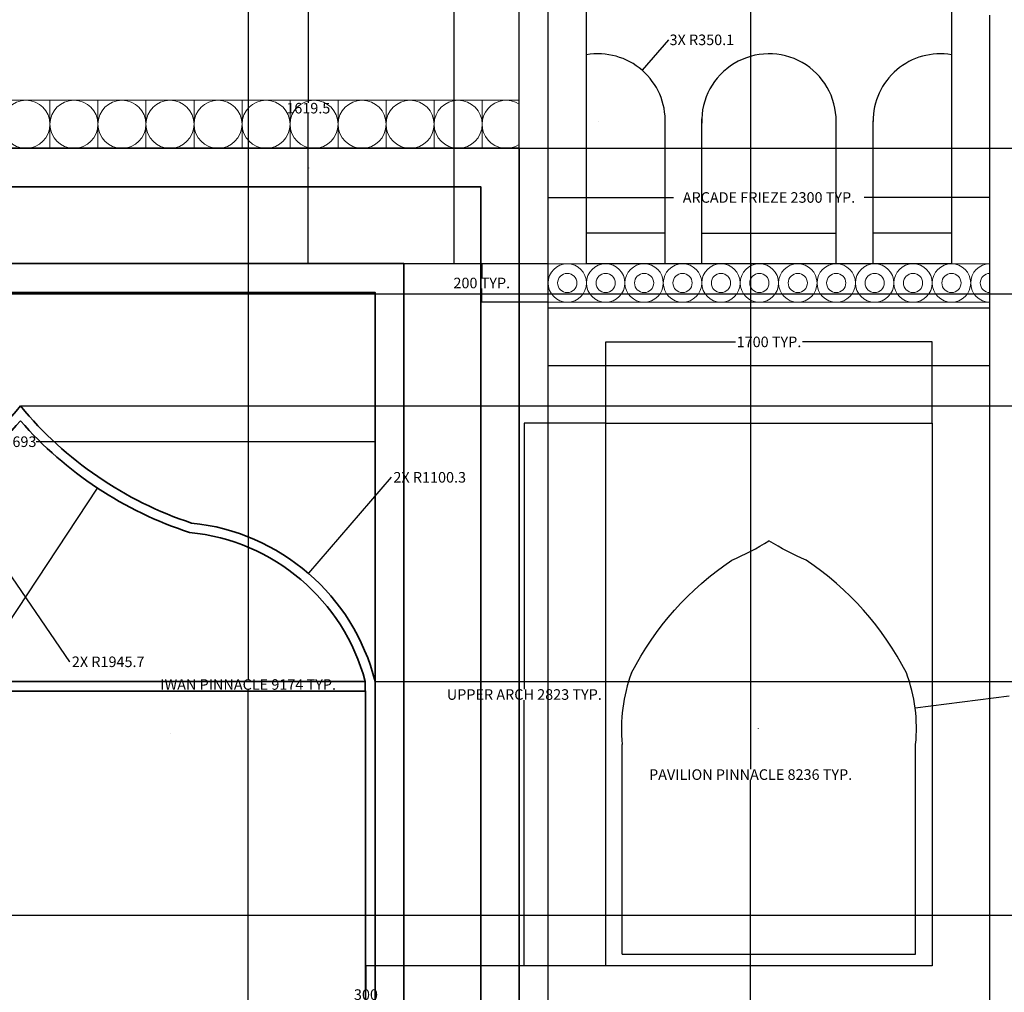
# Model space of a CAD drawing. Units: millimetres. Extents: x 8570 to 49085, y 3782 to 24863.
# Tile 6 of 15: x 22404 to 27529, y 10208 to 15269. Entities that reach past the tile are written whole.
import ezdxf

# ---------------------------------------------------------------- set-up
doc = ezdxf.new("R2010")
doc.units = ezdxf.units.MM
doc.header["$MEASUREMENT"] = 0
doc.header["$PDMODE"] = 3
for name, color, linetype, lineweight in [('A-ANNO-DIMS', 2, 'Continuous', 18), ('A-ELEV', 7, 'Continuous', 25), ('A-ELEV-ARCH', 7, 'Continuous', 25), ('A-ELEV-IWAN', 7, 'Continuous', 35), ('A-ELEV-ORNM', 7, 'Continuous', 13), ('A-ELEV-PIER', 7, 'Continuous', 25), ('A-ROOF-CHAT', 7, 'Continuous', 25)]:
    doc.layers.add(name, color=color, linetype=linetype, lineweight=lineweight)
doc.styles.get("Standard").update_dxf_attribs({"font": 'arial.ttf'})
doc.dimstyles.get("Standard").update_dxf_attribs({"dimtxt": 55, "dimasz": 0.18, "dimexe": 0.18, "dimexo": 0.0625, "dimgap": 0.09, "dimtad": 0, "dimtih": 1, "dimtoh": 1, "dimdec": 0, "dimzin": 0, "dimdsep": 46, "dimtxsty": 'Standard', "dimcen": 0.09, "dimadec": 0, "dimazin": 0, "dimtfac": 1, "dimtdec": 0, "dimtofl": 0, "dimtmove": 0, "dimatfit": 3, "dimfxl": 1, "dimtolj": 1, "dimtzin": 0, "dimarcsym": 0})

# ---------------------------------------------------------------- blocks, each defined once
blk = doc.blocks.new('IWAN-EDGE-PINNACLE')
for p, q in [((35, 0), (35, 9004.5)), ((185, 0), (185, 9004.5))]:
    blk.add_line(p, q)
blk = doc.blocks.new('PAVILION-EDGE-PINNACLE')
for q in [(10, 8069.5), (10, 6246.5)]:
    blk.add_line((10, 0), q)
blk = doc.blocks.new('ARCADE-RING-FRIEZE')
for p, q in [((0, 200), (2300, 200)), ((2300, 200), (2100, 200)), ((0, 0), (2300, 0))]:
    blk.add_line(p, q)
for centre, radius in [((100, 100), 100), ((300, 100), 100), ((500, 100), 100), ((700, 100), 100), ((900, 100), 100), ((1100, 100), 100), ((1300, 100), 100), ((1500, 100), 100), ((1700, 100), 100), ((1900, 100), 100), ((2100, 100), 100), ((100, 100), 50), ((300, 100), 50), ((500, 100), 50), ((700, 100), 50), ((900, 100), 50), ((1100, 100), 50), ((1300, 100), 50), ((1500, 100), 50), ((1700, 100), 50), ((1900, 100), 50), ((2100, 100), 50)]:
    blk.add_circle(centre, radius)
for radius in [100, 50]:
    blk.add_arc((2300, 100), radius, 90, 270)
blk = doc.blocks.new('CHHATRI-ELEV')
for p, q in [((1107.1, 3111.9), (1194.6, 3111.9)), ((819.3, 2507.3), (1150, 2958.1)), ((967.4, 2449.5), (1150, 2958.1)), ((1480.7, 2507.3), (1150, 2958.1)), ((1339.8, 2454.2), (1150, 2958.1)), ((200, 1639.5), (2100, 1639.5)), ((2300, 1569.5), (2300, 1619.5)), ((200, 1549.5), (2100, 1549.5)), ((610, 0), (610, 754)), ((800, 0), (800, 754)), ((1500, 0), (1500, 744.5)), ((1692, 0), (1692, 744.5)), ((610, 158.5), (200, 158.5)), ((800, 158.5), (1500, 158.5)), ((2100, 158.5), (1692, 158.5))]:
    blk.add_line(p, q)
for points in [[(1199.3, 3183.7, 0.216309), (1151.6, 3264, 0.244698), (1103.6, 3171.4, 0.244698)], [(1198.5, 3007.8, 0.216309), (1150.8, 3088.1, 0.244698), (1102.8, 2995.4, 0.244698)], [(259.6, 2102.5, -0.128405), (908.9, 2832.4, 0.03556), (1150, 2958.1)], [(2040.4, 2102.5, 0.128405), (1391.1, 2832.4, -0.03556), (1150, 2958.1)]]:
    blk.add_lwpolyline(points, format="xyb")
for points in [[(225.8, 1639.5, 0.520567), (200.9, 1667.5, 0.520567)], [(273.9, 1639.5, 0.520567), (249, 1667.5, 0.520567)], [(321.9, 1639.5, 0.520567), (297.1, 1667.5, 0.520567)], [(370, 1639.5, 0.520567), (345.1, 1667.5, 0.520567)], [(418, 1639.5, 0.520567), (393.2, 1667.5, 0.520567)], [(466.1, 1639.5, 0.520567), (441.2, 1667.5, 0.520567)], [(514.2, 1639.5, 0.520567), (489.3, 1667.5, 0.520567)], [(562.2, 1639.5, 0.520567), (537.3, 1667.5, 0.520567)], [(610.3, 1639.5, 0.520567), (585.4, 1667.5, 0.520567)], [(658.3, 1639.5, 0.520567), (633.4, 1667.5, 0.520567)], [(706.4, 1639.5, 0.520567), (681.5, 1667.5, 0.520567)], [(754.4, 1639.5, 0.520567), (729.6, 1667.5, 0.520567)], [(802.5, 1639.5, 0.520567), (777.6, 1667.5, 0.520567)], [(850.5, 1639.5, 0.520567), (825.7, 1667.5, 0.520567)], [(898.6, 1639.5, 0.520567), (873.7, 1667.5, 0.520567)], [(946.7, 1639.5, 0.520567), (921.8, 1667.5, 0.520567)], [(994.7, 1639.5, 0.520567), (969.8, 1667.5, 0.520567)], [(1042.8, 1639.5, 0.520567), (1017.9, 1667.5, 0.520567)], [(1090.8, 1639.5, 0.520567), (1065.9, 1667.5, 0.520567)], [(1138.9, 1639.5, 0.520567), (1114, 1667.5, 0.520567)], [(1186.9, 1639.5, 0.520567), (1162.1, 1667.5, 0.520567)], [(1235, 1639.5, 0.520567), (1210.1, 1667.5, 0.520567)], [(1283, 1639.5, 0.520567), (1258.2, 1667.5, 0.520567)], [(1331.1, 1639.5, 0.520567), (1306.2, 1667.5, 0.520567)], [(1379.2, 1639.5, 0.520567), (1354.3, 1667.5, 0.520567)], [(1427.2, 1639.5, 0.520567), (1402.3, 1667.5, 0.520567)], [(1475.3, 1639.5, 0.520567), (1450.4, 1667.5, 0.520567)], [(1523.3, 1639.5, 0.520567), (1498.4, 1667.5, 0.520567)], [(1571.4, 1639.5, 0.520567), (1546.5, 1667.5, 0.520567)], [(1619.4, 1639.5, 0.520567), (1594.6, 1667.5, 0.520567)], [(1667.5, 1639.5, 0.520567), (1642.6, 1667.5, 0.520567)], [(1715.6, 1639.5, 0.520567), (1690.7, 1667.5, 0.520567)], [(1763.6, 1639.5, 0.520567), (1738.7, 1667.5, 0.520567)], [(1811.7, 1639.5, 0.520567), (1786.8, 1667.5, 0.520567)], [(1859.7, 1639.5, 0.520567), (1834.8, 1667.5, 0.520567)], [(1907.8, 1639.5, 0.520567), (1882.9, 1667.5, 0.520567)], [(1955.8, 1639.5, 0.520567), (1931, 1667.5, 0.520567)], [(2003.9, 1639.5, 0.520567), (1979, 1667.5, 0.520567)], [(2051.9, 1639.5, 0.520567), (2027.1, 1667.5, 0.520567)], [(2100, 1639.5, 0.520567), (2075.1, 1667.5, 0.520567)]]:
    blk.add_lwpolyline(points, format="xyb", close=True)
for points in [[(200, 1569.5), (0, 1569.5), (0, 1619.5), (2300, 1619.5), (2300, 1569.5), (2100, 1569.5)], [(2100, 0), (200, 0), (200, 1569.5), (2100, 1569.5), (2100, 0)]]:
    blk.add_lwpolyline(points)
blk.add_circle((1150.8, 3100), 11.9)
for centre, radius, start, end in [((1150.8, 3182.5), 48.5, 193.3065, 1.388), ((1150.8, 3079.7), 54.3, 36.3748, 143.6252), ((1150, 3006.6), 48.5, 193.3065, 1.388), ((1145, 3123.8), 717.3, 225.1557, 315.3968), ((1145, 3123.8), 697.3, 225.1557, 315.3968), ((1217.2, 1743.8), 1022.5, 159.4655, 185.8543), ((1082.8, 1743.8), 1022.5, 354.1457, 20.5345), ((260.1, 742.6), 350.1, 358.1332, 99.8832), ((1149.9, 742.6), 350.1, 359.6883, 181.8668), ((2042.1, 742.6), 350.1, 80.4789, 180.3117)]:
    blk.add_arc(centre, radius, start, end)
blk = doc.blocks.new('WING-UPPER-ARCH')
for p, q in [((86.6, 60), (86.6, 1151.7)), ((1613.4, 60), (1613.4, 1151.7)), ((86.6, 60), (1613.4, 60))]:
    blk.add_line(p, q)
blk.add_lwpolyline([(0, 0), (0, 2823.2), (1700, 2823.2), (1700, 0)], close=True)
for points in [[(134.5, 1523.8, -0.128405), (656.2, 2110.4, 0.03556), (850, 2211.4)], [(1565.5, 1523.8, 0.128405), (1043.8, 2110.4, -0.03556), (850, 2211.4)]]:
    blk.add_lwpolyline(points, format="xyb")
for centre, start, end in [((904, 1235.6), 159.4655, 185.8543), ((796, 1235.6), 354.1457, 20.5345)]:
    blk.add_arc(centre, 821.7, start, end)
blk = doc.blocks.new('IWAN-FRIEZE-ROUNDEL')
blk.add_lwpolyline([(250, 0), (250, 250)])
blk.add_circle((125, 125), 125)
blk = doc.blocks.new('*D19')
at = {"layer": 'A-ANNO-DIMS', "color": 0, "lineweight": -2, "transparency": 16777216}
for p, q in [((24968.9, 16396.4), (23592.7, 16396.4)), ((23592.9, 16396.2), (23592.9, 11838)), ((23592.9, 7222.7), (23592.9, 11780.9)), ((24968.9, 7222.5), (23592.7, 7222.5))]:
    blk.add_line(p, q, dxfattribs=at)
at = {"layer": 'A-ANNO-DIMS', "color": 0, "transparency": 16777216}
for points in [[(23592.9, 16396.2), (23593, 16396.2), (23592.9, 16396.4)], [(23592.9, 7222.7), (23593, 7222.7), (23592.9, 7222.5)]]:
    blk.add_solid(points, dxfattribs=at)
at = {"layer": 'Defpoints', "color": 0, "transparency": 16777216}
for p in [(23592.9, 16396.4), (24969, 16396.4), (24969, 7222.5)]:
    blk.add_point(p, dxfattribs=at)
at = {"layer": 'A-ANNO-DIMS', "color": 0, "transparency": 16777216, "insert": (23592.9, 11809.4), "char_height": 55, "attachment_point": 5}
blk.add_mtext('\\A1;IWAN PINNACLE 9174 TYP.', dxfattribs=at)
blk = doc.blocks.new('*D21')
at = {"layer": 'A-ANNO-DIMS', "color": 0, "lineweight": -2, "transparency": 16777216}
for p, q in [((27443.9, 15458.8), (26208.4, 15458.8)), ((26208.5, 15458.7), (26208.5, 11369.2)), ((26208.5, 7222.7), (26208.5, 11312.1)), ((27443.9, 7222.5), (26208.4, 7222.5))]:
    blk.add_line(p, q, dxfattribs=at)
at = {"layer": 'A-ANNO-DIMS', "color": 0, "transparency": 16777216}
for points in [[(26208.5, 15458.7), (26208.6, 15458.7), (26208.5, 15458.8)], [(26208.5, 7222.7), (26208.6, 7222.7), (26208.5, 7222.5)]]:
    blk.add_solid(points, dxfattribs=at)
at = {"layer": 'Defpoints', "color": 0, "transparency": 16777216}
for p in [(26208.5, 15458.8), (27444, 15458.8), (27444, 7222.5)]:
    blk.add_point(p, dxfattribs=at)
at = {"layer": 'A-ANNO-DIMS', "color": 0, "transparency": 16777216, "insert": (26208.5, 11340.7), "char_height": 55, "attachment_point": 5}
blk.add_mtext('\\A1;PAVILION PINNACLE 8236 TYP.', dxfattribs=at)
blk = doc.blocks.new('*D25')
at = {"layer": 'A-ANNO-DIMS', "color": 0, "lineweight": -2, "transparency": 16777216}
for p, q in [((25153.9, 17263), (24664.2, 17263)), ((24664.4, 17262.9), (24664.4, 15659.6)), ((24664.4, 13999.2), (24664.4, 15602.5)), ((25153.9, 13999), (24664.2, 13999))]:
    blk.add_line(p, q, dxfattribs=at)
at = {"layer": 'A-ANNO-DIMS', "color": 0, "transparency": 16777216}
for points in [[(24664.4, 17262.9), (24664.4, 17262.9), (24664.4, 17263)], [(24664.4, 13999.2), (24664.4, 13999.2), (24664.4, 13999)]]:
    blk.add_solid(points, dxfattribs=at)
at = {"layer": 'Defpoints', "color": 0, "transparency": 16777216}
for p in [(24664.4, 17263), (25154, 17263), (25154, 13999)]:
    blk.add_point(p, dxfattribs=at)
at = {"layer": 'A-ANNO-DIMS', "color": 0, "transparency": 16777216, "insert": (24664.4, 15631), "char_height": 55, "attachment_point": 5}
blk.add_mtext('\\A1;CHHATRI 3264 TYP.', dxfattribs=at)
blk = doc.blocks.new('*D27')
at = {"layer": 'A-ANNO-DIMS', "color": 0, "lineweight": -2, "transparency": 16777216}
for p, q in [((25453.9, 13169), (25030.3, 13169)), ((25030.5, 13168.8), (25030.5, 11785.9)), ((25030.5, 10345.9), (25030.5, 11728.8)), ((25453.9, 10345.8), (25030.3, 10345.8))]:
    blk.add_line(p, q, dxfattribs=at)
at = {"layer": 'A-ANNO-DIMS', "color": 0, "transparency": 16777216}
for points in [[(25030.5, 13168.8), (25030.5, 13168.8), (25030.5, 13169)], [(25030.5, 10345.9), (25030.5, 10345.9), (25030.5, 10345.8)]]:
    blk.add_solid(points, dxfattribs=at)
at = {"layer": 'Defpoints', "color": 0, "transparency": 16777216}
for p in [(25030.5, 13169), (25454, 13169), (25454, 10345.8)]:
    blk.add_point(p, dxfattribs=at)
at = {"layer": 'A-ANNO-DIMS', "color": 0, "transparency": 16777216, "insert": (25030.5, 11757.4), "char_height": 55, "attachment_point": 5}
blk.add_mtext('\\A1;UPPER ARCH 2823 TYP.', dxfattribs=at)
blk = doc.blocks.new('*D28')
at = {"layer": 'A-ANNO-DIMS', "color": 0, "lineweight": -2, "transparency": 16777216}
for p, q in [((25454, 13169.1), (25454, 13592.7)), ((25454.2, 13592.5), (26129.9, 13592.5)), ((27153.8, 13592.5), (26478.1, 13592.5)), ((27154, 13169.1), (27154, 13592.7))]:
    blk.add_line(p, q, dxfattribs=at)
at = {"layer": 'A-ANNO-DIMS', "color": 0, "transparency": 16777216}
for points in [[(25454.2, 13592.5), (25454.2, 13592.5), (25454, 13592.5)], [(27153.8, 13592.5), (27153.8, 13592.5), (27154, 13592.5)]]:
    blk.add_solid(points, dxfattribs=at)
at = {"layer": 'Defpoints', "color": 0, "transparency": 16777216}
for p in [(27154, 13592.5), (25454, 13169), (27154, 13169)]:
    blk.add_point(p, dxfattribs=at)
at = {"layer": 'A-ANNO-DIMS', "color": 0, "transparency": 16777216, "insert": (26304, 13592.5), "char_height": 55, "attachment_point": 5}
blk.add_mtext('\\A1;1700 TYP.', dxfattribs=at)
blk = doc.blocks.new('*D33')
at = {"layer": 'A-ANNO-DIMS', "color": 0, "lineweight": -2, "transparency": 16777216}
for p, q in [((25154, 13999.1), (25154, 14344.2)), ((25154.2, 14344), (25807.7, 14344)), ((27453.8, 14344), (26800.3, 14344)), ((27454, 13999.1), (27454, 14344.2))]:
    blk.add_line(p, q, dxfattribs=at)
at = {"layer": 'A-ANNO-DIMS', "color": 0, "transparency": 16777216}
for points in [[(25154.2, 14344), (25154.2, 14344), (25154, 14344)], [(27453.8, 14344), (27453.8, 14344), (27454, 14344)]]:
    blk.add_solid(points, dxfattribs=at)
at = {"layer": 'Defpoints', "color": 0, "transparency": 16777216}
for p in [(27454, 14344), (25154, 13999), (27454, 13999)]:
    blk.add_point(p, dxfattribs=at)
at = {"layer": 'A-ANNO-DIMS', "color": 0, "transparency": 16777216, "insert": (26304, 14344), "char_height": 55, "attachment_point": 5}
blk.add_mtext('\\A1;ARCADE FRIEZE 2300 TYP.', dxfattribs=at)
blk = doc.blocks.new('*D34')
at = {"layer": 'A-ANNO-DIMS', "color": 0, "lineweight": -2, "transparency": 16777216}
for p, q in [((25153.9, 13999), (24808.8, 13999)), ((24809, 13998.8), (24809, 13927.2)), ((24809, 13799.2), (24809, 13870.8)), ((25153.9, 13799), (24808.8, 13799))]:
    blk.add_line(p, q, dxfattribs=at)
at = {"layer": 'A-ANNO-DIMS', "color": 0, "transparency": 16777216}
for points in [[(24809, 13998.8), (24809, 13998.8), (24809, 13999)], [(24809, 13799.2), (24809, 13799.2), (24809, 13799)]]:
    blk.add_solid(points, dxfattribs=at)
at = {"layer": 'Defpoints', "color": 0, "transparency": 16777216}
for p in [(24809, 13999), (25154, 13999), (25154, 13799)]:
    blk.add_point(p, dxfattribs=at)
at = {"layer": 'A-ANNO-DIMS', "color": 0, "transparency": 16777216, "insert": (24809, 13899), "char_height": 55, "attachment_point": 5}
blk.add_mtext('\\A1;200 TYP.', dxfattribs=at)
blk = doc.blocks.new('*D47')
at = {"layer": 'A-ANNO-DIMS', "color": 0, "lineweight": -2, "transparency": 16777216}
for p, q in [((19811, 14600.1), (19811, 15848.2)), ((19811.2, 15848), (22325.3, 15848)), ((25003.8, 15848), (22489.7, 15848)), ((25004, 14600.1), (25004, 15848.2))]:
    blk.add_line(p, q, dxfattribs=at)
at = {"layer": 'A-ANNO-DIMS', "color": 0, "transparency": 16777216}
for points in [[(19811.2, 15848), (19811.2, 15848), (19811, 15848)], [(25003.8, 15848), (25003.8, 15848), (25004, 15848)]]:
    blk.add_solid(points, dxfattribs=at)
at = {"layer": 'Defpoints', "color": 0, "transparency": 16777216}
for p in [(25004, 15848), (19811, 14600), (25004, 14600)]:
    blk.add_point(p, dxfattribs=at)
at = {"layer": 'A-ANNO-DIMS', "color": 0, "transparency": 16777216, "insert": (22407.5, 15848), "char_height": 55, "attachment_point": 5}
blk.add_mtext('\\A1;5193', dxfattribs=at)
blk = doc.blocks.new('*D48')
at = {"layer": 'A-ANNO-DIMS', "color": 0, "lineweight": -2, "transparency": 16777216}
for p, q in [((20561, 11825.1), (20561, 13073.2)), ((20561.2, 13073), (22325.3, 13073)), ((24253.8, 13073), (22489.7, 13073)), ((24254, 11825.1), (24254, 13073.2))]:
    blk.add_line(p, q, dxfattribs=at)
at = {"layer": 'A-ANNO-DIMS', "color": 0, "transparency": 16777216}
for points in [[(20561.2, 13073), (20561.2, 13073), (20561, 13073)], [(24253.8, 13073), (24253.8, 13073), (24254, 13073)]]:
    blk.add_solid(points, dxfattribs=at)
at = {"layer": 'Defpoints', "color": 0, "transparency": 16777216}
for p in [(24254, 13073), (20561, 11825), (24254, 11825)]:
    blk.add_point(p, dxfattribs=at)
at = {"layer": 'A-ANNO-DIMS', "color": 0, "transparency": 16777216, "insert": (22407.5, 13073), "char_height": 55, "attachment_point": 5}
blk.add_mtext('\\A1;3693', dxfattribs=at)
blk = doc.blocks.new('*D50')
at = {"layer": 'A-ANNO-DIMS', "color": 0, "lineweight": -2, "transparency": 16777216}
for p, q in [((22407.6, 13259), (36055.2, 13259)), ((36055, 13258.8), (36055, 12570.2)), ((36055, 11825.2), (36055, 12513.8)), ((24254.1, 11825), (36055.2, 11825))]:
    blk.add_line(p, q, dxfattribs=at)
at = {"layer": 'A-ANNO-DIMS', "color": 0, "transparency": 16777216}
for points in [[(36055, 13258.8), (36055, 13258.8), (36055, 13259)], [(36055, 11825.2), (36055, 11825.2), (36055, 11825)]]:
    blk.add_solid(points, dxfattribs=at)
at = {"layer": 'Defpoints', "color": 0, "transparency": 16777216}
for p in [(22407.5, 13259), (36055, 13259), (24254, 11825)]:
    blk.add_point(p, dxfattribs=at)
at = {"layer": 'A-ANNO-DIMS', "color": 0, "transparency": 16777216, "insert": (36055, 12542), "char_height": 55, "attachment_point": 5}
blk.add_mtext('\\A1;1434', dxfattribs=at)
blk = doc.blocks.new('*D51')
at = {"layer": 'A-ANNO-DIMS', "color": 0, "lineweight": -2, "transparency": 16777216}
for p, q in [((25004.1, 14600), (36055.2, 14600)), ((36055, 14599.8), (36055, 13957.7)), ((36055, 13259.2), (36055, 13901.3)), ((22407.6, 13259), (36055.2, 13259))]:
    blk.add_line(p, q, dxfattribs=at)
at = {"layer": 'A-ANNO-DIMS', "color": 0, "transparency": 16777216}
for points in [[(36055, 14599.8), (36055, 14599.8), (36055, 14600)], [(36055, 13259.2), (36055, 13259.2), (36055, 13259)]]:
    blk.add_solid(points, dxfattribs=at)
at = {"layer": 'Defpoints', "color": 0, "transparency": 16777216}
for p in [(25004, 14600), (36055, 14600), (22407.5, 13259)]:
    blk.add_point(p, dxfattribs=at)
at = {"layer": 'A-ANNO-DIMS', "color": 0, "transparency": 16777216, "insert": (36055, 13929.5), "char_height": 55, "attachment_point": 5}
blk.add_mtext('\\A1;1341', dxfattribs=at)
blk = doc.blocks.new('*D59')
at = {"layer": 'A-ANNO-DIMS', "color": 0, "lineweight": -2, "transparency": 16777216}
for p, q in [((32990.4, 10606.5), (8684.3, 10606.5)), ((8684.5, 10606.3), (8684.5, 8942.7)), ((8684.5, 7222.7), (8684.5, 8886.3)), ((32870.9, 7222.5), (8684.3, 7222.5))]:
    blk.add_line(p, q, dxfattribs=at)
at = {"layer": 'A-ANNO-DIMS', "color": 0, "transparency": 16777216}
for points in [[(8684.5, 10606.3), (8684.5, 10606.3), (8684.5, 10606.5)], [(8684.5, 7222.7), (8684.5, 7222.7), (8684.5, 7222.5)]]:
    blk.add_solid(points, dxfattribs=at)
at = {"layer": 'Defpoints', "color": 0, "transparency": 16777216}
for p in [(8684.5, 10606.5), (32990.5, 10606.5), (32871, 7222.5)]:
    blk.add_point(p, dxfattribs=at)
at = {"layer": 'A-ANNO-DIMS', "color": 0, "transparency": 16777216, "insert": (8684.5, 8914.5), "char_height": 55, "attachment_point": 5}
blk.add_mtext('\\A1;3384', dxfattribs=at)
blk = doc.blocks.new('*D60')
at = {"layer": 'A-ANNO-DIMS', "color": 0, "lineweight": -2, "transparency": 16777216}
for p, q in [((33041.4, 13840.5), (8684.3, 13840.5)), ((8684.5, 13840.3), (8684.5, 12251.7)), ((8684.5, 10606.7), (8684.5, 12195.3)), ((32990.4, 10606.5), (8684.3, 10606.5))]:
    blk.add_line(p, q, dxfattribs=at)
at = {"layer": 'A-ANNO-DIMS', "color": 0, "transparency": 16777216}
for points in [[(8684.5, 13840.3), (8684.5, 13840.3), (8684.5, 13840.5)], [(8684.5, 10606.7), (8684.5, 10606.7), (8684.5, 10606.5)]]:
    blk.add_solid(points, dxfattribs=at)
at = {"layer": 'Defpoints', "color": 0, "transparency": 16777216}
for p in [(8684.5, 13840.5), (33041.5, 13840.5), (32990.5, 10606.5)]:
    blk.add_point(p, dxfattribs=at)
at = {"layer": 'A-ANNO-DIMS', "color": 0, "transparency": 16777216, "insert": (8684.5, 12223.5), "char_height": 55, "attachment_point": 5}
blk.add_mtext('\\A1;3234', dxfattribs=at)
blk = doc.blocks.new('*D61')
at = {"layer": 'A-ANNO-DIMS', "color": 0, "lineweight": -2, "transparency": 16777216}
for p, q in [((33091.4, 17974), (8684.3, 17974)), ((8684.5, 17973.8), (8684.5, 15935.4)), ((8684.5, 13840.7), (8684.5, 15879.1)), ((33041.4, 13840.5), (8684.3, 13840.5))]:
    blk.add_line(p, q, dxfattribs=at)
at = {"layer": 'A-ANNO-DIMS', "color": 0, "transparency": 16777216}
for points in [[(8684.5, 17973.8), (8684.5, 17973.8), (8684.5, 17974)], [(8684.5, 13840.7), (8684.5, 13840.7), (8684.5, 13840.5)]]:
    blk.add_solid(points, dxfattribs=at)
at = {"layer": 'Defpoints', "color": 0, "transparency": 16777216}
for p in [(8684.5, 17974), (33091.5, 17974), (33041.5, 13840.5)]:
    blk.add_point(p, dxfattribs=at)
at = {"layer": 'A-ANNO-DIMS', "color": 0, "transparency": 16777216, "insert": (8684.5, 15907.2), "char_height": 55, "attachment_point": 5}
blk.add_mtext('\\A1;4133.5', dxfattribs=at)
blk = doc.blocks.new('*D66')
at = {"layer": 'A-ANNO-DIMS', "color": 0, "lineweight": -2, "transparency": 16777216}
for p, q in [((25453.9, 10345.8), (24205.8, 10345.8)), ((24206, 10345.6), (24206, 10223.9)), ((24206, 10045.9), (24206, 10167.6)), ((25453.9, 10045.8), (24205.8, 10045.8))]:
    blk.add_line(p, q, dxfattribs=at)
at = {"layer": 'A-ANNO-DIMS', "color": 0, "transparency": 16777216}
for points in [[(24206, 10345.6), (24206, 10345.6), (24206, 10345.8)], [(24206, 10045.9), (24206, 10045.9), (24206, 10045.8)]]:
    blk.add_solid(points, dxfattribs=at)
at = {"layer": 'Defpoints', "color": 0, "transparency": 16777216}
for p in [(24206, 10345.8), (25454, 10345.8), (25454, 10045.8)]:
    blk.add_point(p, dxfattribs=at)
at = {"layer": 'A-ANNO-DIMS', "color": 0, "transparency": 16777216, "insert": (24206, 10195.7), "char_height": 55, "attachment_point": 5}
blk.add_mtext('\\A1;300', dxfattribs=at)
blk = doc.blocks.new('*D69')
at = {"layer": 'A-ANNO-DIMS', "color": 0, "lineweight": -2, "transparency": 16777216}
for p, q in [((25153.9, 15618.5), (23905.8, 15618.5)), ((23906, 15618.3), (23906, 14836.9)), ((23906, 13999.2), (23906, 14780.6)), ((25153.9, 13999), (23905.8, 13999))]:
    blk.add_line(p, q, dxfattribs=at)
at = {"layer": 'A-ANNO-DIMS', "color": 0, "transparency": 16777216}
for points in [[(23906, 15618.3), (23906, 15618.3), (23906, 15618.5)], [(23906, 13999.2), (23906, 13999.2), (23906, 13999)]]:
    blk.add_solid(points, dxfattribs=at)
at = {"layer": 'Defpoints', "color": 0, "transparency": 16777216}
for p in [(23906, 15618.5), (25154, 15618.5), (25154, 13999)]:
    blk.add_point(p, dxfattribs=at)
at = {"layer": 'A-ANNO-DIMS', "color": 0, "transparency": 16777216, "insert": (23906, 14808.7), "char_height": 55, "attachment_point": 5}
blk.add_mtext('\\A1;1619.5', dxfattribs=at)
blk = doc.blocks.new('*D81')
at = {"layer": 'A-ANNO-DIMS', "color": 0, "lineweight": -2, "transparency": 16777216}
for p, q in [((23908.1, 14497.3), (23908.1, 14497.5)), ((23908.1, 14497.4), (23908.2, 14497.4)), ((22149.1, 11832.6), (22808.6, 12831.7)), ((22148.9, 11832.6), (22149.1, 11832.6))]:
    blk.add_line(p, q, dxfattribs=at)
at = {"layer": 'A-ANNO-DIMS', "color": 0, "transparency": 16777216}
blk.add_solid([(22808.6, 12831.8), (22808.7, 12831.7), (22808.7, 12831.9)], dxfattribs=at)
at = {"layer": 'Defpoints', "color": 0, "transparency": 16777216}
for p in [(23908.1, 14497.4), (22808.7, 12831.9)]:
    blk.add_point(p, dxfattribs=at)
at = {"layer": 'A-ANNO-DIMS', "color": 0, "transparency": 16777216, "insert": (21948.8, 11832.6), "char_height": 55, "attachment_point": 5}
blk.add_mtext('\\A1;2X R1995.7', dxfattribs=at)
blk = doc.blocks.new('*D82')
at = {"layer": 'A-ANNO-DIMS', "color": 0, "lineweight": -2, "transparency": 16777216}
for p, q in [((20906.8, 14497.4), (20906.9, 14497.4)), ((20906.9, 14497.3), (20906.9, 14497.5)), ((22664, 11927.6), (22005.2, 12891.2)), ((22664.2, 11927.6), (22664, 11927.6))]:
    blk.add_line(p, q, dxfattribs=at)
at = {"layer": 'A-ANNO-DIMS', "color": 0, "transparency": 16777216}
blk.add_solid([(22005.2, 12891.2), (22005.1, 12891.1), (22005.1, 12891.3)], dxfattribs=at)
at = {"layer": 'Defpoints', "color": 0, "transparency": 16777216}
for p in [(20906.9, 14497.4), (22005.1, 12891.3)]:
    blk.add_point(p, dxfattribs=at)
at = {"layer": 'A-ANNO-DIMS', "color": 0, "transparency": 16777216, "insert": (22864.3, 11927.6), "char_height": 55, "attachment_point": 5}
blk.add_mtext('\\A1;2X R1945.7', dxfattribs=at)
blk = doc.blocks.new('*D83')
at = {"layer": 'A-ANNO-DIMS', "color": 0, "lineweight": -2, "transparency": 16777216}
for p, q in [((24337.7, 12887.7), (23906.4, 12388.1)), ((24337.9, 12887.7), (24337.7, 12887.7)), ((23187.2, 11555), (23187.4, 11555)), ((23187.3, 11554.9), (23187.3, 11555.1))]:
    blk.add_line(p, q, dxfattribs=at)
at = {"layer": 'A-ANNO-DIMS', "color": 0, "transparency": 16777216}
blk.add_solid([(23906.4, 12388.1), (23906.4, 12388.1), (23906.3, 12387.9)], dxfattribs=at)
at = {"layer": 'Defpoints', "color": 0, "transparency": 16777216}
for p in [(23906.3, 12387.9), (23187.3, 11555)]:
    blk.add_point(p, dxfattribs=at)
at = {"layer": 'A-ANNO-DIMS', "color": 0, "transparency": 16777216, "insert": (24538, 12887.7), "char_height": 55, "attachment_point": 5}
blk.add_mtext('\\A1;2X R1100.3', dxfattribs=at)
blk = doc.blocks.new('*D88')
at = {"layer": 'A-ANNO-DIMS', "color": 0, "lineweight": -2, "transparency": 16777216}
for p, q in [((27554, 11749.3), (27065.2, 11686.3)), ((26249.9, 11581.3), (26250.1, 11581.3)), ((26250, 11581.2), (26250, 11581.4))]:
    blk.add_line(p, q, dxfattribs=at)
at = {"layer": 'A-ANNO-DIMS', "color": 0, "transparency": 16777216}
blk.add_solid([(27065.2, 11686.3), (27065.2, 11686.3), (27065, 11686.3)], dxfattribs=at)
at = {"layer": 'Defpoints', "color": 0, "transparency": 16777216}
for p in [(27065, 11686.3), (26250, 11581.3)]:
    blk.add_point(p, dxfattribs=at)
at = {"layer": 'A-ANNO-DIMS', "color": 0, "transparency": 16777216, "insert": (27732.4, 11749.3), "char_height": 55, "attachment_point": 5}
blk.add_mtext('\\A1;6X R821.7', dxfattribs=at)
blk = doc.blocks.new('*D91')
at = {"layer": 'A-ANNO-DIMS', "color": 0, "lineweight": -2, "transparency": 16777216}
for p, q in [((25781.5, 15164.4), (25643.9, 15006)), ((25781.7, 15164.4), (25781.5, 15164.4)), ((25414, 14741.6), (25414.2, 14741.6)), ((25414.1, 14741.5), (25414.1, 14741.7))]:
    blk.add_line(p, q, dxfattribs=at)
at = {"layer": 'A-ANNO-DIMS', "color": 0, "transparency": 16777216}
blk.add_solid([(25643.8, 15006), (25643.9, 15006), (25643.7, 15005.8)], dxfattribs=at)
at = {"layer": 'Defpoints', "color": 0, "transparency": 16777216}
for p in [(25643.7, 15005.8), (25414.1, 14741.6)]:
    blk.add_point(p, dxfattribs=at)
at = {"layer": 'A-ANNO-DIMS', "color": 0, "transparency": 16777216, "insert": (25954.7, 15164.4), "char_height": 55, "attachment_point": 5}
blk.add_mtext('\\A1;3X R350.1', dxfattribs=at)

msp = doc.modelspace()

# ---------------------------------------------------------------- linework, layer by layer
at = {"layer": 'A-ELEV'}
for p, q in [((25154, 13769), (27454, 13769)), ((25154, 13469), (27454, 13469))]:
    msp.add_line(p, q, dxfattribs=at)
at = {"layer": 'A-ELEV-IWAN'}
msp.add_line((24202.34, 11825), (24202.34, 11775), dxfattribs=at)
for points in [[(19811, 7222.5), (19811, 14600), (25004, 14600), (25004, 7222.5)], [(20011, 7222.5), (20011, 14400), (24804, 14400), (24804, 7222.5)], [(20411, 7222.5), (20411, 14000), (24404, 14000), (24404, 7222.5)], [(20561, 7222.5), (20561, 13850), (24254, 13850), (24254, 7222.5)], [(24254, 7222.5), (24254, 13850)], [(24202.34, 11825), (20611, 11825)], [(24204, 7222.5), (24204, 11775), (20611, 11775)]]:
    msp.add_lwpolyline(points, dxfattribs=at)
for points in [[(20561, 11825, -0.3152594), (21516.4, 12649.7, 0.1414807), (22407.5, 13259)], [(24254, 11825, 0.3152594), (23298.6, 12649.7, -0.1414807), (22407.5, 13259)], [(20612.66, 11825, -0.3133456), (21526.79, 12600.48, 0.1345914), (22407.5, 13181.84, 0.1345914)], [(24202.34, 11825, 0.3133456), (23288.21, 12600.48, -0.1345914), (22407.5, 13181.84, -0.1345914)]]:
    msp.add_lwpolyline(points, format="xyb", dxfattribs=at)
at = {"layer": 'A-ELEV-ORNM'}
msp.add_line((19811, 14850), (25004, 14850), dxfattribs=at)
msp.add_arc((24936, 14725), 125, 57.04365, 302.95635, dxfattribs=at)

# ---------------------------------------------------------------- block references
at = {"layer": 'A-ELEV-ARCH'}
msp.add_blockref('WING-UPPER-ARCH', (25454, 10345.75), dxfattribs=at)
at = {"layer": 'A-ELEV-ORNM'}
for name, p in [('IWAN-FRIEZE-ROUNDEL', (22311, 14600)), ('IWAN-FRIEZE-ROUNDEL', (22561, 14600)), ('IWAN-FRIEZE-ROUNDEL', (22811, 14600)), ('IWAN-FRIEZE-ROUNDEL', (23061, 14600)), ('IWAN-FRIEZE-ROUNDEL', (23311, 14600)), ('IWAN-FRIEZE-ROUNDEL', (23561, 14600)), ('IWAN-FRIEZE-ROUNDEL', (23811, 14600)), ('IWAN-FRIEZE-ROUNDEL', (24061, 14600)), ('IWAN-FRIEZE-ROUNDEL', (24311, 14600)), ('IWAN-FRIEZE-ROUNDEL', (24561, 14600)), ('ARCADE-RING-FRIEZE', (25154, 13799))]:
    msp.add_blockref(name, p, dxfattribs=at)
at = {"layer": 'A-ELEV-PIER'}
for name, p in [('IWAN-EDGE-PINNACLE', (24969, 7222.5)), ('PAVILION-EDGE-PINNACLE', (27444, 7222.5))]:
    msp.add_blockref(name, p, dxfattribs=at)
at = {"layer": 'A-ROOF-CHAT'}
msp.add_blockref('CHHATRI-ELEV', (25154, 13999), dxfattribs=at)

# ---------------------------------------------------------------- dimensions: what is measured, and where the dimension line sits
at = {"layer": 'A-ANNO-DIMS'}
for base, p1, p2, override, picture, middle in [((8684.5, 17974), (33041.5, 13840.5), (33091.5, 17974), {"dimdec": 1, "dimlfac": 1, "dimrnd": 0, "dimzin": 0, "dimdsep": 46, "dimlunit": 2}, '*D61', (8684.5, 15907.25)), ((23906, 15618.5), (25154, 13999), (25154, 15618.5), {"dimdec": 1, "dimlfac": 1, "dimrnd": 0, "dimzin": 0, "dimdsep": 46, "dimlunit": 2}, '*D69', (23906, 14808.75)), ((36055, 14600), (22407.5, 13259), (25004, 14600), {"dimdec": 0, "dimlfac": 1, "dimrnd": 0, "dimzin": 0, "dimdsep": 46, "dimlunit": 2}, '*D51', (36055, 13929.5)), ((8684.5, 13840.5), (32990.5, 10606.5), (33041.5, 13840.5), {"dimdec": 0, "dimlfac": 1, "dimrnd": 0, "dimzin": 0, "dimdsep": 46, "dimlunit": 2}, '*D60', (8684.5, 12223.5)), ((36055, 13259), (24254, 11825), (22407.5, 13259), {"dimdec": 0, "dimlfac": 1, "dimrnd": 0, "dimzin": 0, "dimdsep": 46, "dimlunit": 2}, '*D50', (36055, 12542)), ((8684.5, 10606.5), (32871, 7222.5), (32990.5, 10606.5), {"dimdec": 0, "dimlfac": 1, "dimrnd": 0, "dimzin": 0, "dimdsep": 46, "dimlunit": 2}, '*D59', (8684.5, 8914.5)), ((24206, 10345.75), (25454, 10045.75), (25454, 10345.75), {"dimdec": 0, "dimlfac": 1, "dimrnd": 0, "dimzin": 0, "dimdsep": 46, "dimlunit": 2}, '*D66', (24206, 10195.75))]:
    dim = msp.add_linear_dim(base=base, p1=p1, p2=p2, angle=90, dimstyle='Standard', override=override, dxfattribs=at)
    dim.commit()
    dim.dimension.update_dxf_attribs({"geometry": picture, "text_midpoint": middle})
for base, p1, p2, text, picture, middle in [((24664.39, 17263.04), (25154, 13999), (25154, 17263.04), 'CHHATRI <> TYP.', '*D25', (24664.39, 15631.02)), ((23592.92, 16396.36), (24969, 7222.5), (24969, 16396.36), 'IWAN PINNACLE <> TYP.', '*D19', (23592.92, 11809.43)), ((26208.55, 15458.84), (27444, 7222.5), (27444, 15458.84), 'PAVILION PINNACLE <> TYP.', '*D21', (26208.55, 11340.67)), ((24809, 13999), (25154, 13799), (25154, 13999), '<> TYP.', '*D34', (24809, 13899)), ((25030.51, 13169), (25454, 10345.75), (25454, 13169), 'UPPER ARCH <> TYP.', '*D27', (25030.51, 11757.37))]:
    dim = msp.add_linear_dim(base=base, p1=p1, p2=p2, angle=90, text=text, dimstyle='Standard', override={"dimdec": 0, "dimlfac": 1, "dimrnd": 0, "dimzin": 0, "dimdsep": 46, "dimlunit": 2}, dxfattribs=at)
    dim.commit()
    dim.dimension.update_dxf_attribs({"geometry": picture, "text_midpoint": middle})
for base, p1, p2, picture, middle in [((25004, 15848), (19811, 14600), (25004, 14600), '*D47', (22407.5, 15848)), ((24254, 13073), (20561, 11825), (24254, 11825), '*D48', (22407.5, 13073))]:
    dim = msp.add_linear_dim(base=base, p1=p1, p2=p2, dimstyle='Standard', override={"dimdec": 0, "dimlfac": 1, "dimrnd": 0, "dimzin": 0, "dimdsep": 46, "dimlunit": 2}, dxfattribs=at)
    dim.commit()
    dim.dimension.update_dxf_attribs({"geometry": picture, "text_midpoint": middle})
for center, mpoint, text, picture, middle in [((25414.09, 14741.6), (25643.74, 15005.85), '3X <>', '*D91', (25954.67, 15164.4)), ((20906.85, 14497.42), (22005.05, 12891.31), '2X <>', '*D82', (22864.29, 11927.65)), ((23908.15, 14497.42), (22808.73, 12831.89), '2X <>', '*D81', (21948.77, 11832.58)), ((23187.31, 11555.02), (23906.29, 12387.95), '2X <>', '*D83', (24538, 12887.71)), ((26249.99, 11581.31), (27064.98, 11686.3), '6X <>', '*D88', (27553.97, 11749.28))]:
    dim = msp.add_radius_dim(center=center, mpoint=mpoint, text=text, dimstyle='Standard', override={"dimdec": 1, "dimlfac": 1, "dimrnd": 0, "dimzin": 0, "dimdsep": 46, "dimlunit": 2}, dxfattribs=at)
    dim.commit()
    dim.dimension.update_dxf_attribs({"geometry": picture, "text_midpoint": middle, "dimtype": 164})
for base, p1, p2, text, picture, middle in [((27454, 14344), (25154, 13999), (27454, 13999), 'ARCADE FRIEZE <> TYP.', '*D33', (26304, 14344)), ((27154, 13592.49), (25454, 13169), (27154, 13169), '<> TYP.', '*D28', (26304, 13592.49))]:
    dim = msp.add_linear_dim(base=base, p1=p1, p2=p2, text=text, dimstyle='Standard', override={"dimdec": 0, "dimlfac": 1, "dimrnd": 0, "dimzin": 0, "dimdsep": 46, "dimlunit": 2}, dxfattribs=at)
    dim.commit()
    dim.dimension.update_dxf_attribs({"geometry": picture, "text_midpoint": middle})

doc.saveas('drawing.dxf')
